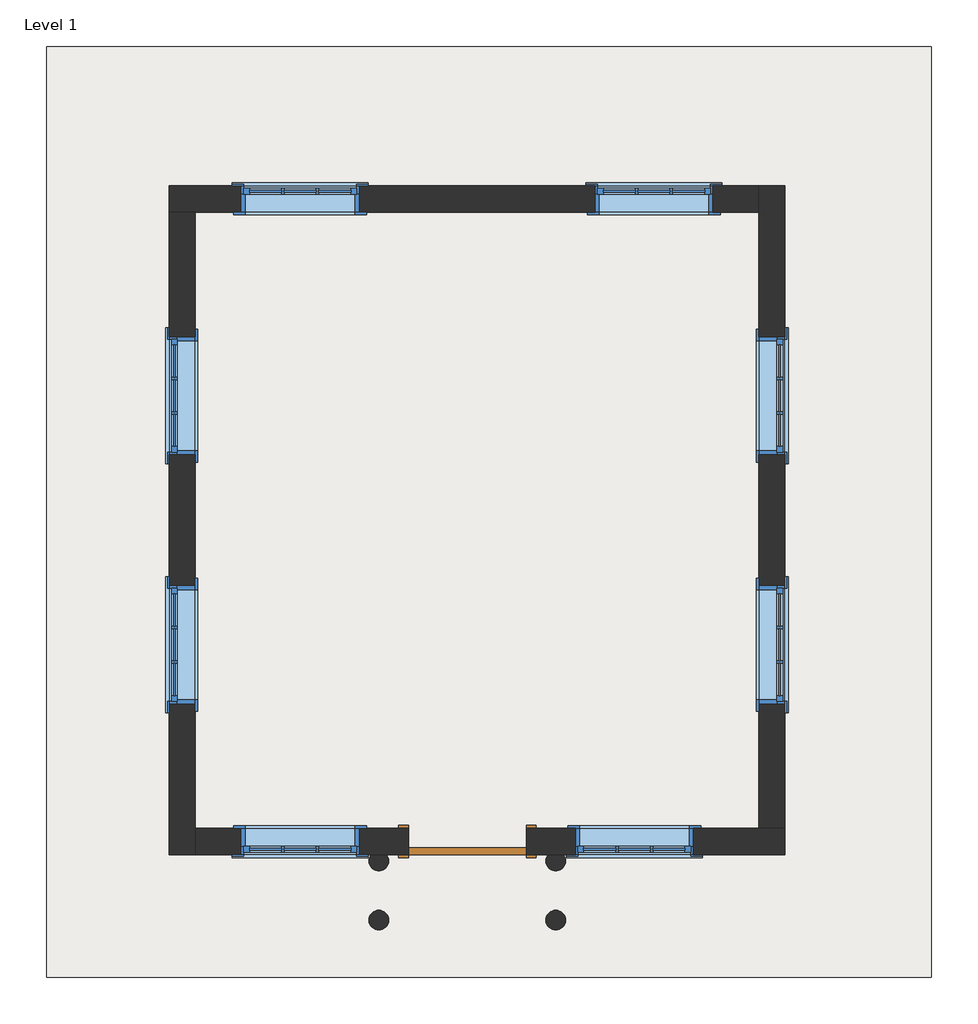
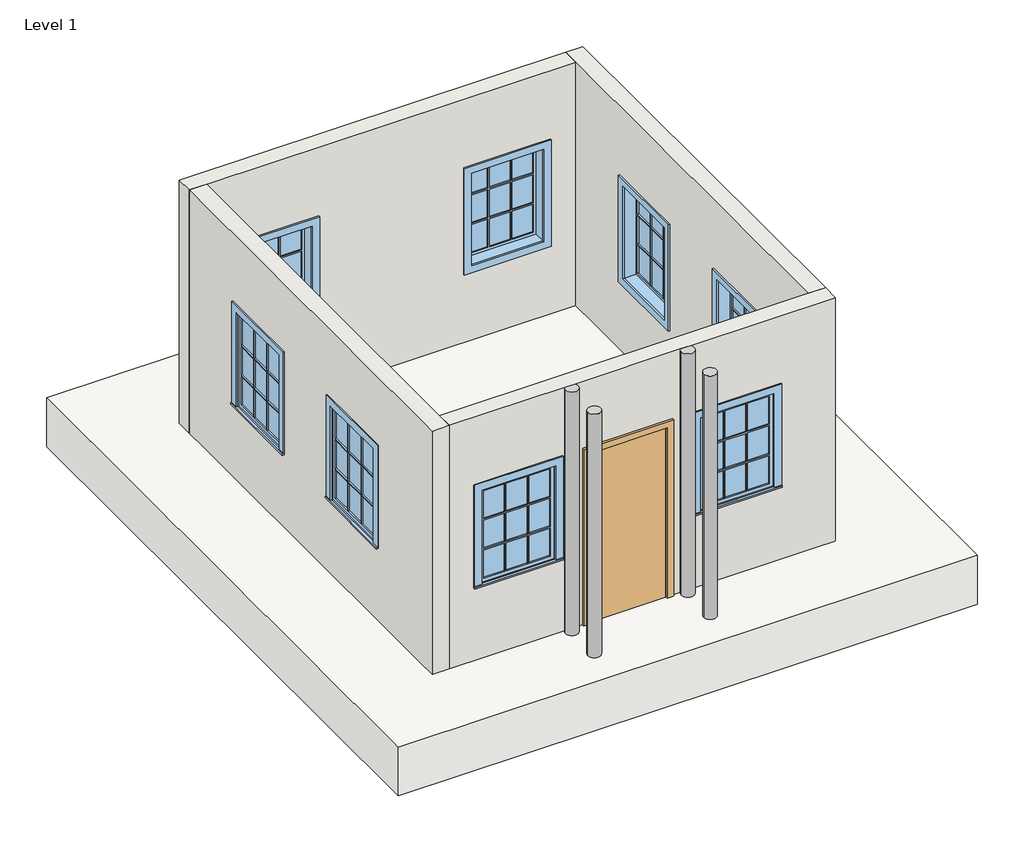
# One storey: 8 windows, 4 columns, 4 walls, 1 door, 1 slab.
"""IFC4 building model written with IfcOpenShell, lengths in millimetres."""

from ifc_helpers import new_model, si_unit, point, frame, frame_2d, origin, origin_with_axes, place, context, project, spatial, polyline, circle_curve, trimmed, segment, composite_curve, outline, extrude, faceted_brep, transform, mapped, element, save
from components import column_79e7fb11, door_54dd4da4, window_29c06734

model = new_model("IFC4")

# Units and contexts
model_context = context("Model", 3, world=origin())
ifc_project = project(units=[si_unit("LENGTHUNIT", "METRE", prefix="MILLI")], contexts=[model_context])

# Site, building, storey
site = spatial("IfcSite", under=ifc_project)
building = spatial("IfcBuilding", under=site)
storey = spatial("IfcBuildingStorey", under=building, Name="Level 1", Elevation=0.0)

# Columns
placement = place(None, origin())
element("IfcColumn", 1, ObjectType="Round Column : 06\" Diameter", at=placement, inside=storey, context=model_context, shape_type="SweptSolid", body=[
    extrude(outline(composite_curve([segment(trimmed(circle_curve(frame_2d((-7988.0670776, -7578.1100774)), 76.2), [point((-7911.8670776, -7578.1100774))], [point((-8064.2670776, -7578.1100774))], False, "CARTESIAN"), True, "CONTINUOUS"), segment(trimmed(circle_curve(frame_2d((-7988.0670776, -7578.1100774)), 76.2), [point((-8064.2670776, -7578.1100774))], [point((-8044.8632042, -7527.3100774))], False, "CARTESIAN"), True, "CONTINUOUS"), segment(polyline([(-8044.8632042, -7527.3100774), (-7931.270951, -7527.3100774)]), True, "CONTINUOUS"), segment(trimmed(circle_curve(frame_2d((-7988.0670776, -7578.1100774)), 76.2), [point((-7931.270951, -7527.3100774))], [point((-7911.8670776, -7578.1100774))], False, "CARTESIAN"), True, "CONTINUOUS")], self_intersect=False)), origin_with_axes(), (0.0, 0.0, 1.0), 3048.0),
])
element("IfcColumn", 2, ObjectType="Round Column : 06\" Diameter", at=placement, inside=storey, context=model_context, shape_type="SweptSolid", body=[
    extrude(outline(composite_curve([segment(trimmed(circle_curve(frame_2d((-6616.4670776, -7578.1100774)), 76.2), [point((-6540.2670776, -7578.1100774))], [point((-6692.6670776, -7578.1100774))], False, "CARTESIAN"), True, "CONTINUOUS"), segment(trimmed(circle_curve(frame_2d((-6616.4670776, -7578.1100774)), 76.2), [point((-6692.6670776, -7578.1100774))], [point((-6673.2632042, -7527.3100774))], False, "CARTESIAN"), True, "CONTINUOUS"), segment(polyline([(-6673.2632042, -7527.3100774), (-6559.670951, -7527.3100774)]), True, "CONTINUOUS"), segment(trimmed(circle_curve(frame_2d((-6616.4670776, -7578.1100774)), 76.2), [point((-6559.670951, -7527.3100774))], [point((-6540.2670776, -7578.1100774))], False, "CARTESIAN"), True, "CONTINUOUS")], self_intersect=False)), origin_with_axes(), (0.0, 0.0, 1.0), 3048.0),
])
column_shape = column_79e7fb11(model_context)
element("IfcColumn", 3, ObjectType="Round Column : 06\" Diameter", at=placement, inside=storey, context=model_context, shape_type="MappedRepresentation", body=[
    mapped(column_shape, transform((-7988.0670776, -8035.3100774, 0.0), x_axis=(1.0, 0.0, 0.0), y_axis=(0.0, 1.0, 0.0), z_axis=(0.0, 0.0, 1.0))),
])
element("IfcColumn", 4, ObjectType="Round Column : 06\" Diameter", at=placement, inside=storey, context=model_context, shape_type="MappedRepresentation", body=[
    mapped(column_shape, transform((-6616.4670776, -8035.3100774, 0.0), x_axis=(1.0, 0.0, 0.0), y_axis=(0.0, 1.0, 0.0), z_axis=(0.0, 0.0, 1.0))),
])

# Door
door_shape = door_54dd4da4(model_context)
element("IfcDoor", 5, ObjectType="Single-Flush : 36\" x 84\"", at=placement, inside=storey, context=model_context, shape_type="MappedRepresentation", body=[
    mapped(door_shape, transform((-7302.2670776, -7425.7100774, 0.0), x_axis=(-1.0, 0.0, 0.0), y_axis=(0.0, -1.0, 0.0), z_axis=(0.0, 0.0, 1.0))),
])

# Slab
element("IfcSlab", 6, ObjectType="Generic - 2'", at=placement, inside=storey, context=model_context, shape_type="SweptSolid", body=[
    extrude(outline(polyline([(-3706.3792677, -1265.8175323), (-3706.3792677, -8479.4175323), (-10564.3792677, -8479.4175323), (-10564.3792677, -1265.8175323), (-3706.3792677, -1265.8175323)])), frame((0.0, 0.0, -609.6), z_axis=(0.0, 0.0, 1.0), x_axis=(1.0, 0.0, 0.0)), (0.0, 0.0, 1.0), 609.6),
])

# Walls
element("IfcWall", 7, ObjectType="Generic - 8\"", at=placement, inside=storey, context=model_context, shape_type="Brep", body=[
    faceted_brep([(-9613.6670776, -2548.9100774, 0.0), (-9410.4670776, -2548.9100774, 0.0), (-5041.6670776, -2548.9100774, 0.0), (-5041.6670776, -2548.9100774, 3048.0), (-9410.4670776, -2548.9100774, 3048.0), (-9613.6670776, -2548.9100774, 3048.0), (-5397.2670776, -2548.9100774, 2133.6), (-5397.2670776, -2548.9100774, 914.4), (-6311.6670776, -2548.9100774, 914.4), (-6311.6670776, -2548.9100774, 2133.6), (-8140.4670776, -2548.9100774, 2133.6), (-8140.4670776, -2548.9100774, 914.4), (-9054.8670776, -2548.9100774, 914.4), (-9054.8670776, -2548.9100774, 2133.6), (-9613.6670776, -2345.7100774, 0.0), (-9613.6670776, -2345.7100774, 3048.0), (-5041.6670776, -2345.7100774, 3048.0), (-5041.6670776, -2345.7100774, 0.0), (-5397.2670776, -2345.7100774, 2133.6), (-6311.6670776, -2345.7100774, 2133.6), (-6311.6670776, -2345.7100774, 914.4), (-5397.2670776, -2345.7100774, 914.4), (-8140.4670776, -2345.7100774, 2133.6), (-9054.8670776, -2345.7100774, 2133.6), (-9054.8670776, -2345.7100774, 914.4), (-8140.4670776, -2345.7100774, 914.4)], [[[0, 1, 2, 3, 4, 5], [6, 7, 8, 9], [10, 11, 12, 13]], [[14, 15, 16, 17], [18, 19, 20, 21], [22, 23, 24, 25]], [[2, 1, 0, 14, 17]], [[5, 4, 3, 16, 15]], [[0, 5, 15, 14]], [[3, 2, 17, 16]], [[7, 6, 18, 21]], [[8, 7, 21, 20]], [[9, 8, 20, 19]], [[6, 9, 19, 18]], [[11, 10, 22, 25]], [[12, 11, 25, 24]], [[13, 12, 24, 23]], [[10, 13, 23, 22]]]),
])
element("IfcWall", 8, ObjectType="Generic - 8\"", at=placement, inside=storey, context=model_context, shape_type="Brep", body=[
    faceted_brep([(-9410.4670776, -7527.3100774, 0.0), (-9410.4670776, -7324.1100774, 0.0), (-9410.4670776, -2548.9100774, 0.0), (-9410.4670776, -2548.9100774, 3048.0), (-9410.4670776, -7324.1100774, 3048.0), (-9410.4670776, -7527.3100774, 3048.0), (-9410.4670776, -3514.1100774, 2133.6), (-9410.4670776, -3514.1100774, 914.4), (-9410.4670776, -4428.5100774, 914.4), (-9410.4670776, -4428.5100774, 2133.6), (-9410.4670776, -5444.5100774, 2133.6), (-9410.4670776, -5444.5100774, 914.4), (-9410.4670776, -6358.9100774, 914.4), (-9410.4670776, -6358.9100774, 2133.6), (-9613.6670776, -7527.3100774, 0.0), (-9613.6670776, -7527.3100774, 3048.0), (-9613.6670776, -2548.9100774, 3048.0), (-9613.6670776, -2548.9100774, 0.0), (-9613.6670776, -3514.1100774, 2133.6), (-9613.6670776, -4428.5100774, 2133.6), (-9613.6670776, -4428.5100774, 914.4), (-9613.6670776, -3514.1100774, 914.4), (-9613.6670776, -5444.5100774, 2133.6), (-9613.6670776, -6358.9100774, 2133.6), (-9613.6670776, -6358.9100774, 914.4), (-9613.6670776, -5444.5100774, 914.4)], [[[0, 1, 2, 3, 4, 5], [6, 7, 8, 9], [10, 11, 12, 13]], [[14, 15, 16, 17], [18, 19, 20, 21], [22, 23, 24, 25]], [[2, 1, 0, 14, 17]], [[5, 4, 3, 16, 15]], [[0, 5, 15, 14]], [[3, 2, 17, 16]], [[7, 6, 18, 21]], [[8, 7, 21, 20]], [[9, 8, 20, 19]], [[6, 9, 19, 18]], [[11, 10, 22, 25]], [[12, 11, 25, 24]], [[13, 12, 24, 23]], [[10, 13, 23, 22]]]),
])
element("IfcWall", 9, ObjectType="Generic - 8\"", at=placement, inside=storey, context=model_context, shape_type="Brep", body=[
    faceted_brep([(-7759.4670776, -7324.1100774, 2133.6), (-7759.4670776, -7324.1100774, 0.0), (-9410.4670776, -7324.1100774, 0.0), (-9410.4670776, -7324.1100774, 3048.0), (-5041.6670776, -7324.1100774, 3048.0), (-4838.4670776, -7324.1100774, 3048.0), (-4838.4670776, -7324.1100774, 0.0), (-5041.6670776, -7324.1100774, 0.0), (-6845.0670776, -7324.1100774, 0.0), (-6845.0670776, -7324.1100774, 2133.6), (-6464.0670776, -7324.1100774, 2133.6), (-6464.0670776, -7324.1100774, 914.4), (-5549.6670776, -7324.1100774, 914.4), (-5549.6670776, -7324.1100774, 2133.6), (-9054.8670776, -7324.1100774, 2133.6), (-9054.8670776, -7324.1100774, 914.4), (-8140.4670776, -7324.1100774, 914.4), (-8140.4670776, -7324.1100774, 2133.6), (-9410.4670776, -7527.3100774, 0.0), (-8044.8632042, -7527.3100774, 0.0), (-7931.270951, -7527.3100774, 0.0), (-7759.4670776, -7527.3100774, 0.0), (-7759.4670776, -7527.3100774, 2133.6), (-6845.0670776, -7527.3100774, 2133.6), (-6845.0670776, -7527.3100774, 0.0), (-6673.2632042, -7527.3100774, 0.0), (-6559.670951, -7527.3100774, 0.0), (-4838.4670776, -7527.3100774, 0.0), (-4838.4670776, -7527.3100774, 3048.0), (-6559.670951, -7527.3100774, 3048.0), (-6673.2632042, -7527.3100774, 3048.0), (-7931.270951, -7527.3100774, 3048.0), (-8044.8632042, -7527.3100774, 3048.0), (-9410.4670776, -7527.3100774, 3048.0), (-6464.0670776, -7527.3100774, 2133.6), (-5549.6670776, -7527.3100774, 2133.6), (-5549.6670776, -7527.3100774, 914.4), (-6464.0670776, -7527.3100774, 914.4), (-9054.8670776, -7527.3100774, 2133.6), (-8140.4670776, -7527.3100774, 2133.6), (-8140.4670776, -7527.3100774, 914.4), (-9054.8670776, -7527.3100774, 914.4)], [[[0, 1, 2, 3, 4, 5, 6, 7, 8, 9], [10, 11, 12, 13], [14, 15, 16, 17]], [[18, 19, 20, 21, 22, 23, 24, 25, 26, 27, 28, 29, 30, 31, 32, 33], [34, 35, 36, 37], [38, 39, 40, 41]], [[2, 1, 21, 20, 19, 18]], [[8, 7, 6, 27, 26, 25, 24]], [[5, 4, 3, 33, 32, 31, 30, 29, 28]], [[6, 5, 28, 27]], [[3, 2, 18, 33]], [[11, 10, 34, 37]], [[12, 11, 37, 36]], [[13, 12, 36, 35]], [[10, 13, 35, 34]], [[15, 14, 38, 41]], [[16, 15, 41, 40]], [[17, 16, 40, 39]], [[14, 17, 39, 38]], [[22, 21, 1, 0]], [[23, 22, 0, 9]], [[24, 23, 9, 8]]]),
])
element("IfcWall", 10, ObjectType="Generic - 8\"", at=placement, inside=storey, context=model_context, shape_type="Brep", body=[
    faceted_brep([(-5041.6670776, -2345.7100774, 0.0), (-5041.6670776, -2548.9100774, 0.0), (-5041.6670776, -7324.1100774, 0.0), (-5041.6670776, -7324.1100774, 3048.0), (-5041.6670776, -2548.9100774, 3048.0), (-5041.6670776, -2345.7100774, 3048.0), (-5041.6670776, -6358.9100774, 2133.6), (-5041.6670776, -6358.9100774, 914.4), (-5041.6670776, -5444.5100774, 914.4), (-5041.6670776, -5444.5100774, 2133.6), (-5041.6670776, -4428.5100774, 2133.6), (-5041.6670776, -4428.5100774, 914.4), (-5041.6670776, -3514.1100774, 914.4), (-5041.6670776, -3514.1100774, 2133.6), (-4838.4670776, -2345.7100774, 0.0), (-4838.4670776, -2345.7100774, 3048.0), (-4838.4670776, -7324.1100774, 3048.0), (-4838.4670776, -7324.1100774, 0.0), (-4838.4670776, -6358.9100774, 2133.6), (-4838.4670776, -5444.5100774, 2133.6), (-4838.4670776, -5444.5100774, 914.4), (-4838.4670776, -6358.9100774, 914.4), (-4838.4670776, -4428.5100774, 2133.6), (-4838.4670776, -3514.1100774, 2133.6), (-4838.4670776, -3514.1100774, 914.4), (-4838.4670776, -4428.5100774, 914.4)], [[[0, 1, 2, 3, 4, 5], [6, 7, 8, 9], [10, 11, 12, 13]], [[14, 15, 16, 17], [18, 19, 20, 21], [22, 23, 24, 25]], [[2, 1, 0, 14, 17]], [[5, 4, 3, 16, 15]], [[0, 5, 15, 14]], [[3, 2, 17, 16]], [[7, 6, 18, 21]], [[8, 7, 21, 20]], [[9, 8, 20, 19]], [[6, 9, 19, 18]], [[11, 10, 22, 25]], [[12, 11, 25, 24]], [[13, 12, 24, 23]], [[10, 13, 23, 22]]]),
])

# Windows
window_shape = window_29c06734(model_context)
element("IfcWindow", 11, ObjectType="Casement 3x3 with Trim : 36\" x 48\"", at=placement, inside=storey, context=model_context, shape_type="MappedRepresentation", body=[
    mapped(window_shape, transform((-4940.0670776, -5901.7100774, 0.0), x_axis=(0.0, -1.0, 0.0), y_axis=(1.0, 0.0, 0.0), z_axis=(0.0, 0.0, 1.0))),
])
element("IfcWindow", 12, ObjectType="Casement 3x3 with Trim : 36\" x 48\"", at=placement, inside=storey, context=model_context, shape_type="MappedRepresentation", body=[
    mapped(window_shape, transform((-4940.0670776, -3971.3100774, 0.0), x_axis=(0.0, -1.0, 0.0), y_axis=(1.0, 0.0, 0.0), z_axis=(0.0, 0.0, 1.0))),
])
element("IfcWindow", 13, ObjectType="Casement 3x3 with Trim : 36\" x 48\"", at=placement, inside=storey, context=model_context, shape_type="MappedRepresentation", body=[
    mapped(window_shape, transform((-6006.8670776, -7425.7100774, 0.0), x_axis=(-1.0, 0.0, 0.0), y_axis=(0.0, -1.0, 0.0), z_axis=(0.0, 0.0, 1.0))),
])
element("IfcWindow", 14, ObjectType="Casement 3x3 with Trim : 36\" x 48\"", at=placement, inside=storey, context=model_context, shape_type="MappedRepresentation", body=[
    mapped(window_shape, transform((-8597.6670776, -7425.7100774, 0.0), x_axis=(-1.0, 0.0, 0.0), y_axis=(0.0, -1.0, 0.0), z_axis=(0.0, 0.0, 1.0))),
])
element("IfcWindow", 15, ObjectType="Casement 3x3 with Trim : 36\" x 48\"", at=placement, inside=storey, context=model_context, shape_type="MappedRepresentation", body=[
    mapped(window_shape, transform((-9512.0670776, -3971.3100774, 0.0), x_axis=(0.0, 1.0, 0.0), y_axis=(-1.0, 0.0, 0.0), z_axis=(0.0, 0.0, 1.0))),
])
element("IfcWindow", 16, ObjectType="Casement 3x3 with Trim : 36\" x 48\"", at=placement, inside=storey, context=model_context, shape_type="MappedRepresentation", body=[
    mapped(window_shape, transform((-9512.0670776, -5901.7100774, 0.0), x_axis=(0.0, 1.0, 0.0), y_axis=(-1.0, 0.0, 0.0), z_axis=(0.0, 0.0, 1.0))),
])
element("IfcWindow", 17, ObjectType="Casement 3x3 with Trim : 36\" x 48\"", at=placement, inside=storey, context=model_context, shape_type="MappedRepresentation", body=[
    mapped(window_shape, transform((-5854.4670776, -2447.3100774, 0.0), x_axis=(1.0, 0.0, 0.0), y_axis=(0.0, 1.0, 0.0), z_axis=(0.0, 0.0, 1.0))),
])
element("IfcWindow", 18, ObjectType="Casement 3x3 with Trim : 36\" x 48\"", at=placement, inside=storey, context=model_context, shape_type="MappedRepresentation", body=[
    mapped(window_shape, transform((-8597.6670776, -2447.3100774, 0.0), x_axis=(1.0, 0.0, 0.0), y_axis=(0.0, 1.0, 0.0), z_axis=(0.0, 0.0, 1.0))),
])

save(model, "model.ifc")

# Revit data of these elements
# Type "Round Column : 06\" Diameter"
#   Assembly Code = "B1010200"
#   Diameter = 0' - 6"
#   Offset Base = 0' - 0"
#   Offset Top = 0' - 0"
#   Material = none
# Type "Single-Flush : 36\" x 84\""
#   Type Mark = "1"
#   Construction Type Id = "MDOOR"
#   Assembly Code = "C1020"
#   Analytic Construction = "Metal"
#   Thickness = 0' - 2"
#   Heat Transfer Coefficient (U) = 0.651978 BTU/(h·ft²·°F)
#   Height = 7' - 0"
#   Trim Projection Ext = 0' - 1"
#   Trim Projection Int = 0' - 1"
#   Trim Width = 0' - 3"
#   Width = 3' - 0"
#   Define Thermal Properties by = 1
#   Door Material = Door - Panel
#   Frame Material = Door - Frame
#   Visual Light Transmittance = 0
#   Solar Heat Gain Coefficient = 0
#   Function = (empty or 0)
#   Wall Closure = (empty or 0)
# Type "Generic - 2'"
#   Assembly Code = "B1010"
#   Function = 0
#   Layers, outside or top first: 2' - 0" no material (function 1)
# Type "Generic - 8\""
#   Assembly Code = "B2010"
#   Layers, outside or top first: 0' - 8" no material (function 1)
# Type "Casement 3x3 with Trim : 36\" x 48\""
#   Type Mark = "10"
#   Construction Type Id = "GSP4R"
#   Assembly Code = "B2020100"
#   Analytic Construction = "1/8 in Pilkington single glazing"
#   Visual Light Transmittance = 0.9
#   Solar Heat Gain Coefficient = 0.78
#   Heat Transfer Coefficient (U) = 0.6496 BTU/(h·ft²·°F)
#   Height = 4' - 0"
#   Default Sill Height = 3' - 0"
#   Trim Projection - Ext. = 0' - 0 1/2"
#   Trim Projection - Int. = 0' - 0 3/4"
#   Trim Width - Exterior = 0' - 3 1/2"
#   Trim Width - Interior = 0' - 3 1/2"
#   Width = 3' - 0"
#   Window Inset = 0' - 0 3/4"
#   Define Thermal Properties by = 1
#   Glass Pane Material = Glass
#   Sash Material = Sash
#   Trim Exterior Material = Trim
#   Trim Interior Material = Trim
#   Wall Closure = (empty or 0)
# Elements 1, 2 (IfcColumn, "Round Column : 06\" Diameter")
#   Phase Created = New Construction
#   Materials on its faces: "Default Wall"
# Elements 3, 4 (IfcColumn, "Round Column : 06\" Diameter")
#   Phase Created = New Construction
# Element 5 (IfcDoor, "Single-Flush : 36\" x 84\"")
#   Phase Created = New Construction
#   Materials on its faces: "Door - Frame", "Door - Panel"
# Element 6 (IfcSlab, "Generic - 2'")
#   Height Offset From Level = 0' - 0"
#   Phase Created = New Construction
#   Materials on its faces: "Default Floor"
# Elements 7, 8, 9, 10 (IfcWall, "Generic - 8\"")
#   Top Offset = 0' - 0"
#   Base Offset = 0' - 0"
#   Unconnected Height = 10' - 0"
#   wall height = 10' - 0"
#   Phase Created = New Construction
#   Base Constraint = Level 1
#   Materials on its faces: "Default Wall"
# Element 11 (IfcWindow, "Casement 3x3 with Trim : 36\" x 48\"")
#   Mark = "9"
#   Phase Created = New Construction
#   Materials on its faces: "Sash", "Glass", "Trim"
# Element 12 (IfcWindow, "Casement 3x3 with Trim : 36\" x 48\"")
#   Mark = "10"
#   Phase Created = New Construction
#   Materials on its faces: "Sash", "Glass", "Trim"
# Element 13 (IfcWindow, "Casement 3x3 with Trim : 36\" x 48\"")
#   Mark = "11"
#   Phase Created = New Construction
#   Materials on its faces: "Sash", "Glass", "Trim"
# Element 14 (IfcWindow, "Casement 3x3 with Trim : 36\" x 48\"")
#   Mark = "12"
#   Phase Created = New Construction
#   Materials on its faces: "Sash", "Glass", "Trim"
# Element 15 (IfcWindow, "Casement 3x3 with Trim : 36\" x 48\"")
#   Mark = "13"
#   Phase Created = New Construction
#   Materials on its faces: "Sash", "Glass", "Trim"
# Element 16 (IfcWindow, "Casement 3x3 with Trim : 36\" x 48\"")
#   Mark = "14"
#   Phase Created = New Construction
#   Materials on its faces: "Sash", "Glass", "Trim"
# Element 17 (IfcWindow, "Casement 3x3 with Trim : 36\" x 48\"")
#   Mark = "15"
#   Phase Created = New Construction
#   Materials on its faces: "Sash", "Glass", "Trim"
# Element 18 (IfcWindow, "Casement 3x3 with Trim : 36\" x 48\"")
#   Mark = "16"
#   Phase Created = New Construction
#   Materials on its faces: "Sash", "Glass", "Trim"
# Materials
#   "Door - Panel": class "Wood", colour RGB 210 159 95, transparency 0
#   "Door - Frame": colour RGB 118 70 51, transparency 0
#   "Glass": class "Glass", colour RGB 0 128 192, transparency 0.75, Description = "Soda Lime Glass", Cost = 0
#   "Sash": class "Wood", colour RGB 224 178 126, transparency 0
#   "Trim": class "Wood", colour RGB 224 178 126, transparency 0
#   "Default Wall": colour RGB 128 128 128, transparency 0
#   "Default Floor": colour RGB 128 128 128, transparency 0
